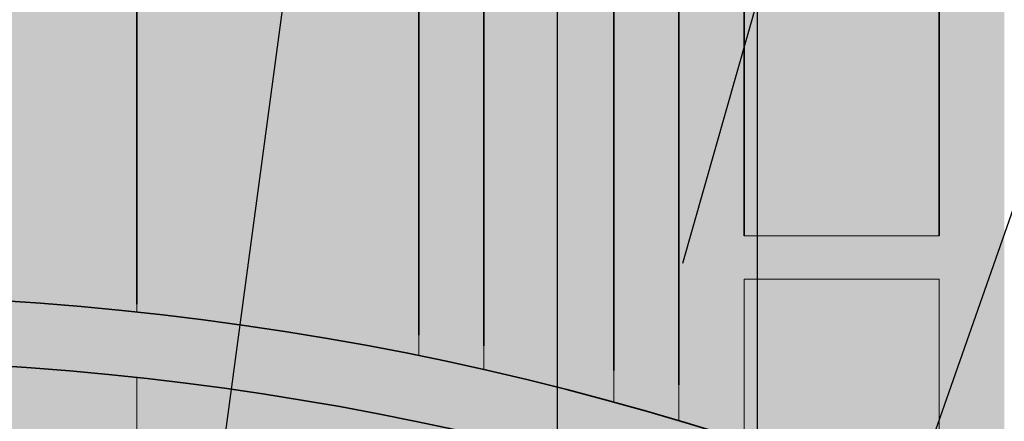
# Model space of a CAD drawing. Units: millimetres. Extents: x 130 to 1021, y 147 to 699.
# Tile 27 of 40: x 442 to 487, y 505 to 524. Entities that reach past the tile are written whole.
import ezdxf

# ---------------------------------------------------------------- set-up
doc = ezdxf.new("R2010")
doc.units = ezdxf.units.MM
doc.header["$MEASUREMENT"] = 0
for name, color, linetype, lineweight in [('A-ANNO-DIMS', 2, 'Continuous', 18), ('A-ELEV', 7, 'Continuous', 35), ('A-ELEV-PATT', 9, 'Continuous', 13), ('A-ELEV-RAIL', 6, 'Continuous', 18)]:
    doc.layers.add(name, color=color, linetype=linetype, lineweight=lineweight)
doc.styles.get("Standard").update_dxf_attribs({"font": 'arial.ttf'})
doc.dimstyles.get("Standard").update_dxf_attribs({"dimtxt": 20, "dimasz": 10, "dimexe": 10, "dimexo": 10, "dimgap": 5, "dimtad": 0, "dimtih": 1, "dimtoh": 1, "dimdec": 0, "dimzin": 0, "dimdsep": 46, "dimtxsty": 'Standard', "dimcen": 5, "dimadec": 0, "dimazin": 0, "dimtfac": 1, "dimtdec": 0, "dimtofl": 0, "dimtmove": 0, "dimatfit": 3, "dimfxl": 1, "dimtolj": 1, "dimtzin": 0, "dimarcsym": 0})

# ---------------------------------------------------------------- blocks, each defined once
blk = doc.blocks.new('*D11')
at = {"layer": 'A-ANNO-DIMS', "color": 0, "lineweight": -2, "transparency": 16777216}
for p, q in [((737.374, 648.699), (737.374, 149.739)), ((299.374, 566.947), (299.374, 149.739)), ((309.374, 159.739), (490.857, 159.739)), ((727.374, 159.739), (545.891, 159.739))]:
    blk.add_line(p, q, dxfattribs=at)
at = {"layer": 'A-ANNO-DIMS', "color": 0, "transparency": 16777216}
for points in [[(309.374, 161.406), (309.374, 158.073), (299.374, 159.739)], [(727.374, 161.406), (727.374, 158.073), (737.374, 159.739)]]:
    blk.add_solid(points, dxfattribs=at)
at = {"layer": 'Defpoints', "color": 0, "transparency": 16777216}
for p in [(737.374, 658.699), (299.374, 576.947), (737.374, 159.739)]:
    blk.add_point(p, dxfattribs=at)
at = {"layer": 'A-ANNO-DIMS', "color": 0, "transparency": 16777216, "insert": (518.374, 159.739), "char_height": 20, "attachment_point": 5}
blk.add_mtext('\\A1;438', dxfattribs=at)
blk = doc.blocks.new('*D12')
at = {"layer": 'A-ANNO-DIMS', "color": 0, "lineweight": -2, "transparency": 16777216}
for p, q in [((477.374, 661.947), (265.074, 661.947)), ((275.074, 651.947), (275.074, 438.205)), ((275.074, 194.039), (275.074, 407.782)), ((357.163, 184.039), (265.074, 184.039))]:
    blk.add_line(p, q, dxfattribs=at)
at = {"layer": 'A-ANNO-DIMS', "color": 0, "transparency": 16777216}
for points in [[(273.407, 651.947), (276.74, 651.947), (275.074, 661.947)], [(273.407, 194.039), (276.74, 194.039), (275.074, 184.039)]]:
    blk.add_solid(points, dxfattribs=at)
at = {"layer": 'Defpoints', "color": 0, "transparency": 16777216}
for p in [(275.074, 661.947), (487.374, 661.947), (367.163, 184.039)]:
    blk.add_point(p, dxfattribs=at)
at = {"layer": 'A-ANNO-DIMS', "color": 0, "transparency": 16777216, "insert": (275.074, 422.993), "char_height": 20, "attachment_point": 5}
blk.add_mtext('\\A1;477.9', dxfattribs=at)
blk = doc.blocks.new('*D16')
at = {"layer": 'A-ANNO-DIMS', "color": 0, "lineweight": -2, "transparency": 16777216}
for p, q in [((357.941, 411.947), (357.941, 696.247)), ((363.922, 579.884), (363.922, 696.247)), ((347.941, 686.247), (337.941, 686.247)), ((373.922, 686.247), (383.922, 686.247))]:
    blk.add_line(p, q, dxfattribs=at)
at = {"layer": 'A-ANNO-DIMS', "color": 0, "transparency": 16777216}
for points in [[(347.941, 687.914), (347.941, 684.581), (357.941, 686.247)], [(373.922, 687.914), (373.922, 684.581), (363.922, 686.247)]]:
    blk.add_solid(points, dxfattribs=at)
at = {"layer": 'Defpoints', "color": 0, "transparency": 16777216}
for p in [(363.922, 686.247), (363.922, 569.884), (357.941, 401.947)]:
    blk.add_point(p, dxfattribs=at)
at = {"layer": 'A-ANNO-DIMS', "color": 0, "transparency": 16777216, "insert": (420.737, 686.247), "char_height": 20, "attachment_point": 5}
blk.add_mtext('\\A1;5.981', dxfattribs=at)
blk = doc.blocks.new('*D17')
at = {"layer": 'A-ANNO-DIMS', "color": 0, "lineweight": -2, "transparency": 16777216}
for p, q in [((363.922, 579.884), (363.922, 696.247)), ((375.85, 490.216), (375.85, 696.247)), ((353.922, 686.247), (343.922, 686.247)), ((385.85, 686.247), (395.85, 686.247))]:
    blk.add_line(p, q, dxfattribs=at)
at = {"layer": 'A-ANNO-DIMS', "color": 0, "transparency": 16777216}
for points in [[(353.922, 687.914), (353.922, 684.581), (363.922, 686.247)], [(385.85, 687.914), (385.85, 684.581), (375.85, 686.247)]]:
    blk.add_solid(points, dxfattribs=at)
at = {"layer": 'Defpoints', "color": 0, "transparency": 16777216}
for p in [(375.85, 686.247), (363.922, 569.884), (375.85, 480.216)]:
    blk.add_point(p, dxfattribs=at)
at = {"layer": 'A-ANNO-DIMS', "color": 0, "transparency": 16777216, "insert": (441.444, 686.247), "char_height": 20, "attachment_point": 5}
blk.add_mtext('\\A1;11.928', dxfattribs=at)
blk = doc.blocks.new('*D18')
at = {"layer": 'A-ANNO-DIMS', "color": 0, "lineweight": -2, "transparency": 16777216}
for p, q in [((375.85, 490.216), (375.85, 696.247)), ((382.374, 388.947), (382.374, 696.247)), ((365.85, 686.247), (355.85, 686.247)), ((392.374, 686.247), (402.374, 686.247))]:
    blk.add_line(p, q, dxfattribs=at)
at = {"layer": 'A-ANNO-DIMS', "color": 0, "transparency": 16777216}
for points in [[(365.85, 687.914), (365.85, 684.581), (375.85, 686.247)], [(392.374, 687.914), (392.374, 684.581), (382.374, 686.247)]]:
    blk.add_solid(points, dxfattribs=at)
at = {"layer": 'Defpoints', "color": 0, "transparency": 16777216}
for p in [(382.374, 686.247), (375.85, 480.216), (382.374, 378.947)]:
    blk.add_point(p, dxfattribs=at)
at = {"layer": 'A-ANNO-DIMS', "color": 0, "transparency": 16777216, "insert": (441.132, 686.247), "char_height": 20, "attachment_point": 5}
blk.add_mtext('\\A1;6.524', dxfattribs=at)
blk = doc.blocks.new('*D19')
at = {"layer": 'A-ANNO-DIMS', "color": 0, "lineweight": -2, "transparency": 16777216}
for p, q in [((382.374, 388.947), (382.374, 696.247)), ((414.652, 510.881), (414.652, 696.247)), ((392.374, 686.247), (404.652, 686.247)), ((414.652, 686.247), (424.652, 686.247))]:
    blk.add_line(p, q, dxfattribs=at)
at = {"layer": 'A-ANNO-DIMS', "color": 0, "transparency": 16777216}
for points in [[(392.374, 687.914), (392.374, 684.581), (382.374, 686.247)], [(404.652, 687.914), (404.652, 684.581), (414.652, 686.247)]]:
    blk.add_solid(points, dxfattribs=at)
at = {"layer": 'Defpoints', "color": 0, "transparency": 16777216}
for p in [(414.652, 686.247), (414.652, 500.881), (382.374, 378.947)]:
    blk.add_point(p, dxfattribs=at)
at = {"layer": 'A-ANNO-DIMS', "color": 0, "transparency": 16777216, "insert": (463.411, 686.247), "char_height": 20, "attachment_point": 5}
blk.add_mtext('\\A1;32.28', dxfattribs=at)
blk = doc.blocks.new('*D20')
at = {"layer": 'A-ANNO-DIMS', "color": 0, "lineweight": -2, "transparency": 16777216}
for p, q in [((414.652, 510.881), (414.652, 696.247)), ((432.374, 388.947), (432.374, 696.247)), ((404.652, 686.247), (394.652, 686.247)), ((442.374, 686.247), (452.374, 686.247))]:
    blk.add_line(p, q, dxfattribs=at)
at = {"layer": 'A-ANNO-DIMS', "color": 0, "transparency": 16777216}
for points in [[(404.652, 687.914), (404.652, 684.581), (414.652, 686.247)], [(442.374, 687.914), (442.374, 684.581), (432.374, 686.247)]]:
    blk.add_solid(points, dxfattribs=at)
at = {"layer": 'Defpoints', "color": 0, "transparency": 16777216}
for p in [(432.374, 686.247), (414.652, 500.881), (432.374, 378.947)]:
    blk.add_point(p, dxfattribs=at)
at = {"layer": 'A-ANNO-DIMS', "color": 0, "transparency": 16777216, "insert": (490.075, 686.247), "char_height": 20, "attachment_point": 5}
blk.add_mtext('\\A1;17.72', dxfattribs=at)
blk = doc.blocks.new('*D21')
at = {"layer": 'A-ANNO-DIMS', "color": 0, "lineweight": -2, "transparency": 16777216}
for p, q in [((432.374, 388.947), (432.374, 696.247)), ((447.374, 656.947), (447.374, 696.247)), ((422.374, 686.247), (412.374, 686.247)), ((457.374, 686.247), (467.374, 686.247))]:
    blk.add_line(p, q, dxfattribs=at)
at = {"layer": 'A-ANNO-DIMS', "color": 0, "transparency": 16777216}
for points in [[(422.374, 687.914), (422.374, 684.581), (432.374, 686.247)], [(457.374, 687.914), (457.374, 684.581), (447.374, 686.247)]]:
    blk.add_solid(points, dxfattribs=at)
at = {"layer": 'Defpoints', "color": 0, "transparency": 16777216}
for p in [(447.374, 686.247), (447.374, 646.947), (432.374, 378.947)]:
    blk.add_point(p, dxfattribs=at)
at = {"layer": 'A-ANNO-DIMS', "color": 0, "transparency": 16777216, "insert": (485.832, 686.247), "char_height": 20, "attachment_point": 5}
blk.add_mtext('\\A1;15', dxfattribs=at)
blk = doc.blocks.new('*D22')
at = {"layer": 'A-ANNO-DIMS', "color": 0, "lineweight": -2, "transparency": 16777216}
for p, q in [((447.374, 656.947), (447.374, 696.247)), ((466.767, 403.947), (466.767, 696.247)), ((437.374, 686.247), (427.374, 686.247)), ((476.767, 686.247), (486.767, 686.247))]:
    blk.add_line(p, q, dxfattribs=at)
at = {"layer": 'A-ANNO-DIMS', "color": 0, "transparency": 16777216}
for points in [[(437.374, 687.914), (437.374, 684.581), (447.374, 686.247)], [(476.767, 687.914), (476.767, 684.581), (466.767, 686.247)]]:
    blk.add_solid(points, dxfattribs=at)
at = {"layer": 'Defpoints', "color": 0, "transparency": 16777216}
for p in [(466.767, 686.247), (447.374, 646.947), (466.767, 393.947)]:
    blk.add_point(p, dxfattribs=at)
at = {"layer": 'A-ANNO-DIMS', "color": 0, "transparency": 16777216, "insert": (532.34, 686.247), "char_height": 20, "attachment_point": 5}
blk.add_mtext('\\A1;19.393', dxfattribs=at)
blk = doc.blocks.new('*D23')
at = {"layer": 'A-ANNO-DIMS', "color": 0, "lineweight": -2, "transparency": 16777216}
for p, q in [((466.767, 403.947), (466.767, 696.247)), ((475.988, 209.039), (475.988, 696.247)), ((456.767, 686.247), (446.767, 686.247)), ((485.988, 686.247), (495.988, 686.247))]:
    blk.add_line(p, q, dxfattribs=at)
at = {"layer": 'A-ANNO-DIMS', "color": 0, "transparency": 16777216}
for points in [[(456.767, 687.914), (456.767, 684.581), (466.767, 686.247)], [(485.988, 687.914), (485.988, 684.581), (475.988, 686.247)]]:
    blk.add_solid(points, dxfattribs=at)
at = {"layer": 'Defpoints', "color": 0, "transparency": 16777216}
for p in [(475.988, 686.247), (466.767, 393.947), (475.988, 199.039)]:
    blk.add_point(p, dxfattribs=at)
at = {"layer": 'A-ANNO-DIMS', "color": 0, "transparency": 16777216, "insert": (534.631, 686.247), "char_height": 20, "attachment_point": 5}
blk.add_mtext('\\A1;9.222', dxfattribs=at)
blk = doc.blocks.new('*D24')
at = {"layer": 'A-ANNO-DIMS', "color": 0, "lineweight": -2, "transparency": 16777216}
for p, q in [((475.988, 209.039), (475.988, 696.247)), ((487.374, 671.947), (487.374, 696.247)), ((465.988, 686.247), (455.988, 686.247)), ((497.374, 686.247), (507.374, 686.247))]:
    blk.add_line(p, q, dxfattribs=at)
at = {"layer": 'A-ANNO-DIMS', "color": 0, "transparency": 16777216}
for points in [[(465.988, 687.914), (465.988, 684.581), (475.988, 686.247)], [(497.374, 687.914), (497.374, 684.581), (487.374, 686.247)]]:
    blk.add_solid(points, dxfattribs=at)
at = {"layer": 'Defpoints', "color": 0, "transparency": 16777216}
for p in [(487.374, 686.247), (487.374, 661.947), (475.988, 199.039)]:
    blk.add_point(p, dxfattribs=at)
at = {"layer": 'A-ANNO-DIMS', "color": 0, "transparency": 16777216, "insert": (553.022, 686.247), "char_height": 20, "attachment_point": 5}
blk.add_mtext('\\A1;11.385', dxfattribs=at)
blk = doc.blocks.new('*D25')
at = {"layer": 'A-ANNO-DIMS', "color": 0, "lineweight": -2, "transparency": 16777216}
for p, q in [((487.374, 671.947), (487.374, 696.247)), ((494.102, 506.908), (494.102, 696.247)), ((477.374, 686.247), (467.374, 686.247)), ((504.102, 686.247), (514.102, 686.247))]:
    blk.add_line(p, q, dxfattribs=at)
at = {"layer": 'A-ANNO-DIMS', "color": 0, "transparency": 16777216}
for points in [[(477.374, 687.914), (477.374, 684.581), (487.374, 686.247)], [(504.102, 687.914), (504.102, 684.581), (494.102, 686.247)]]:
    blk.add_solid(points, dxfattribs=at)
at = {"layer": 'Defpoints', "color": 0, "transparency": 16777216}
for p in [(494.102, 686.247), (487.374, 661.947), (494.102, 496.908)]:
    blk.add_point(p, dxfattribs=at)
at = {"layer": 'A-ANNO-DIMS', "color": 0, "transparency": 16777216, "insert": (552.922, 686.247), "char_height": 20, "attachment_point": 5}
blk.add_mtext('\\A1;6.728', dxfattribs=at)
blk = doc.blocks.new('*D26')
at = {"layer": 'A-ANNO-DIMS', "color": 0, "lineweight": -2, "transparency": 16777216}
for p, q in [((494.102, 506.908), (494.102, 696.247)), ((502.374, 593.947), (502.374, 696.247)), ((484.102, 686.247), (474.102, 686.247)), ((512.374, 686.247), (522.374, 686.247))]:
    blk.add_line(p, q, dxfattribs=at)
at = {"layer": 'A-ANNO-DIMS', "color": 0, "transparency": 16777216}
for points in [[(484.102, 687.914), (484.102, 684.581), (494.102, 686.247)], [(512.374, 687.914), (512.374, 684.581), (502.374, 686.247)]]:
    blk.add_solid(points, dxfattribs=at)
at = {"layer": 'Defpoints', "color": 0, "transparency": 16777216}
for p in [(502.374, 686.247), (502.374, 583.947), (494.102, 496.908)]:
    blk.add_point(p, dxfattribs=at)
at = {"layer": 'A-ANNO-DIMS', "color": 0, "transparency": 16777216, "insert": (561.03, 686.247), "char_height": 20, "attachment_point": 5}
blk.add_mtext('\\A1;8.272', dxfattribs=at)
blk = doc.blocks.new('*D65')
at = {"layer": 'A-ANNO-DIMS', "color": 0, "lineweight": -2, "transparency": 16777216}
for p, q in [((495.463, 509.127), (472.508, 423.108)), ((505.463, 509.127), (495.463, 509.127)), ((427.374, 248.979), (427.374, 258.979)), ((422.374, 253.979), (432.374, 253.979))]:
    blk.add_line(p, q, dxfattribs=at)
at = {"layer": 'A-ANNO-DIMS', "color": 0, "transparency": 16777216}
blk.add_solid([(470.898, 423.538), (474.118, 422.679), (469.93, 413.447)], dxfattribs=at)
at = {"layer": 'Defpoints', "color": 0, "transparency": 16777216}
for p in [(469.93, 413.447), (427.374, 253.979)]:
    blk.add_point(p, dxfattribs=at)
at = {"layer": 'A-ANNO-DIMS', "color": 0, "transparency": 16777216, "insert": (561.623, 509.127), "char_height": 20, "attachment_point": 5}
blk.add_mtext('\\A1;R165.05', dxfattribs=at)
blk = doc.blocks.new('*D67')
at = {"layer": 'A-ANNO-DIMS', "color": 0, "lineweight": -2, "transparency": 16777216}
for p, q in [((479.756, 492.431), (462.144, 412.223)), ((489.756, 492.431), (479.756, 492.431)), ((427.07, 247.496), (427.07, 257.496)), ((422.07, 252.496), (432.07, 252.496))]:
    blk.add_line(p, q, dxfattribs=at)
at = {"layer": 'A-ANNO-DIMS', "color": 0, "transparency": 16777216}
blk.add_solid([(460.516, 412.58), (463.772, 411.865), (459.999, 402.455)], dxfattribs=at)
at = {"layer": 'Defpoints', "color": 0, "transparency": 16777216}
for p in [(459.999, 402.455), (427.07, 252.496)]:
    blk.add_point(p, dxfattribs=at)
at = {"layer": 'A-ANNO-DIMS', "color": 0, "transparency": 16777216, "insert": (545.841, 492.431), "char_height": 20, "attachment_point": 5}
blk.add_mtext('\\A1;R153.53', dxfattribs=at)
blk = doc.blocks.new('*D69')
at = {"layer": 'A-ANNO-DIMS', "color": 0, "lineweight": -2, "transparency": 16777216}
for p, q in [((507.746, 572.261), (483.091, 501.813)), ((517.746, 572.261), (507.746, 572.261)), ((433.191, 354.23), (433.191, 364.23)), ((428.191, 359.23), (438.191, 359.23))]:
    blk.add_line(p, q, dxfattribs=at)
at = {"layer": 'A-ANNO-DIMS', "color": 0, "transparency": 16777216}
blk.add_solid([(481.518, 502.363), (484.664, 501.262), (479.788, 492.374)], dxfattribs=at)
at = {"layer": 'Defpoints', "color": 0, "transparency": 16777216}
for p in [(479.788, 492.374), (433.191, 359.23)]:
    blk.add_point(p, dxfattribs=at)
at = {"layer": 'A-ANNO-DIMS', "color": 0, "transparency": 16777216, "insert": (573.824, 572.261), "char_height": 20, "attachment_point": 5}
blk.add_mtext('\\A1;R141.06', dxfattribs=at)
blk = doc.blocks.new('*D71')
at = {"layer": 'A-ANNO-DIMS', "color": 0, "lineweight": -2, "transparency": 16777216}
for p, q in [((492.108, 581.609), (472.542, 512.666)), ((502.108, 581.609), (492.108, 581.609)), ((432.65, 367.109), (432.65, 377.109)), ((427.65, 372.109), (437.65, 372.109))]:
    blk.add_line(p, q, dxfattribs=at)
at = {"layer": 'A-ANNO-DIMS', "color": 0, "transparency": 16777216}
blk.add_solid([(470.938, 513.121), (474.145, 512.211), (469.812, 503.046)], dxfattribs=at)
at = {"layer": 'Defpoints', "color": 0, "transparency": 16777216}
for p in [(469.812, 503.046), (432.65, 372.109)]:
    blk.add_point(p, dxfattribs=at)
at = {"layer": 'A-ANNO-DIMS', "color": 0, "transparency": 16777216, "insert": (548.493, 581.609), "char_height": 20, "attachment_point": 5}
blk.add_mtext('\\A1;R136.1', dxfattribs=at)
blk = doc.blocks.new('*D72')
at = {"layer": 'A-ANNO-DIMS', "color": 0, "lineweight": -2, "transparency": 16777216}
for p, q in [((460.658, 573.64), (451.279, 503.49)), ((470.658, 573.64), (460.658, 573.64)), ((432.115, 355.142), (432.115, 365.142)), ((427.115, 360.142), (437.115, 360.142))]:
    blk.add_line(p, q, dxfattribs=at)
at = {"layer": 'A-ANNO-DIMS', "color": 0, "transparency": 16777216}
blk.add_solid([(449.628, 503.711), (452.931, 503.27), (449.954, 493.579)], dxfattribs=at)
at = {"layer": 'Defpoints', "color": 0, "transparency": 16777216}
for p in [(449.954, 493.579), (432.115, 360.142)]:
    blk.add_point(p, dxfattribs=at)
at = {"layer": 'A-ANNO-DIMS', "color": 0, "transparency": 16777216, "insert": (526.64, 573.64), "char_height": 20, "attachment_point": 5}
blk.add_mtext('\\A1;R134.62', dxfattribs=at)

msp = doc.modelspace()

# ---------------------------------------------------------------- hatches: boundary and pattern name
at = {"layer": 'A-ELEV-PATT'}
h = msp.add_hatch(color=256, dxfattribs=at)
h.dxf.hatch_style = 1
h.paths.add_polyline_path([(737.3738, 658.6988, 0.0135961), (632.4019, 661.9473), (607.3738, 661.9473), (487.3738, 661.9473), (487.3738, 649.9473), (607.3738, 649.9473), (632.3794, 649.9473, -0.0136841), (737.3738, 646.6784)])
h.paths.add_polyline_path([(732.3738, 643.9599, 0.0130529), (632.3738, 646.9473), (607.3738, 646.9473), (487.3738, 646.9473), (487.3738, 596.9473), (632.3738, 596.9473, -0.0130529), (732.3738, 593.9599)])
h.paths.add_polyline_path([(737.3738, 593.6732, 0.0137063), (632.3738, 596.9473), (487.3738, 596.9473), (487.3738, 586.9473), (632.355, 586.9473, -0.0137808), (737.3738, 583.6559)])
h.paths.add_polyline_path([(447.3738, 646.9473), (307.3738, 646.9473), (302.3738, 646.9473), (302.3738, 634.9473), (447.3738, 634.9473)])
h.paths.add_polyline_path([(447.3738, 631.9473), (307.3738, 631.9473), (307.3738, 586.9473), (447.3738, 586.9473)])
h.paths.add_polyline_path([(447.3738, 586.9473), (307.3738, 586.9473), (302.3738, 586.9473), (302.3738, 576.9473), (447.3738, 576.9473)])
h.paths.add_polyline_path([(447.3738, 573.9473), (367.3738, 573.9473), (367.3738, 539.9473), (447.3738, 539.9473)])
h.paths.add_polyline_path([(447.3738, 537.9473), (367.3738, 537.9473), (367.3738, 507.9473), (400.392, 507.4253, -0.001728), (401.3281, 507.6451, -0.5220025), (425.6117, 511.0391, -0.0391849), (447.3738, 510.4359), (447.3738, 510.7883)])
h.paths.add_polyline_path([(394.7238, 505.9473), (367.3738, 505.9473), (367.3738, 476.9473, -0.0146512), (375.8501, 480.2159), (376.1506, 499.2266, -0.0355419)])
h.paths.add_polyline_path([(632.3738, 583.9473), (552.3738, 583.9473), (552.3738, 550.9473), (632.3738, 550.9473)])
h.paths.add_polyline_path([(632.3738, 548.9473), (552.3738, 548.9473), (552.3738, 515.9473), (632.3738, 515.9473)])
h.paths.add_polyline_path([(632.3738, 513.9473), (552.3738, 513.9473), (552.3738, 476.9473), (632.3738, 476.9473)])
h.paths.add_polyline_path([(737.3738, 473.6903, 0.0136326), (632.3926, 476.9473), (552.3738, 476.9473), (487.3738, 476.9473), (487.3738, 466.9473), (632.3738, 466.9473, -0.0137063), (737.3738, 463.6732)])
h.paths.add_polyline_path([(732.3738, 460.9552, 0.0130741), (632.3681, 463.9473), (487.3738, 463.9473), (487.3738, 407.735, -0.0032286), (489.3544, 406.9473), (632.3926, 406.9473, -0.0129826), (732.3738, 403.9755)])
h.paths.add_polyline_path([(487.3738, 463.9473, 0.20133), (367.3738, 463.9473), (367.3738, 407.735, -0.1882031), (487.3738, 407.735)])
h.paths.add_polyline_path([(367.3738, 476.9473), (367.3738, 466.9473, -0.2013309), (487.3738, 466.9473), (487.3738, 476.9473, 0.20133)])
h.paths.add_polyline_path([(367.3738, 463.9473), (307.3738, 463.9473), (307.3738, 401.9473), (357.9413, 401.9473), (367.3738, 407.735)])
h.paths.add_polyline_path([(367.3738, 476.9473), (302.3738, 476.9473), (302.3738, 466.9473), (367.3738, 466.9473)])
h.paths.add_polyline_path([(632.8184, 366.9453), (552.3738, 366.9453), (552.3738, 393.9473), (632.8184, 393.9473)])
h.paths.add_polyline_path([(632.8184, 357.2114), (632.8184, 363.9453), (552.3738, 363.9453), (552.3738, 357.2114), (552.3738, 336.9453), (632.8184, 336.9453)])
h.paths.add_polyline_path([(632.8184, 333.9453), (552.3738, 333.9453), (552.3738, 306.9453), (632.8184, 306.9453)])
h.paths.add_polyline_path([(632.8184, 303.9453), (552.3738, 303.9453), (552.3738, 273.9473), (632.355, 273.9473, 0.0000608), (632.8184, 273.9491)])
h.paths.add_polyline_path([(737.3738, 403.6903, 0.0136326), (632.3926, 406.9473), (489.3544, 406.9473, 0.1915481), (367.3738, 407.735), (367.3738, 396.9473, -0.2013309), (487.3738, 396.9473), (632.3738, 396.9473, -0.0137063), (737.3738, 393.6732)])
h.paths.add_polyline_path([(357.9413, 401.9473), (307.3738, 401.9473), (307.3738, 391.9473), (357.9413, 391.9473)])
h.paths.add_polyline_path([(357.9413, 357.2114), (357.9413, 388.9473), (307.3738, 388.9473), (307.3738, 357.2114), (307.3738, 273.9473), (357.9413, 273.9473)])
h.paths.add_polyline_path([(732.3738, 263.93, -0.0130317), (632.3794, 260.9473), (466.7667, 260.9473), (466.7667, 240.9473), (469.8406, 236.978), (469.8406, 221.978), (472.9145, 218.0087), (472.9145, 213.9473), (607.3738, 213.9473), (732.3738, 213.9473)])
h.paths.add_polyline_path([(732.3738, 290.889), (722.479, 290.889), (722.479, 301.889), (732.3738, 301.889), (732.3738, 305.889), (722.479, 305.889), (722.479, 316.889), (732.3738, 316.889), (732.3738, 320.889), (722.479, 320.889), (722.479, 331.889), (732.3738, 331.889), (732.3738, 335.889), (722.479, 335.889), (722.479, 346.889), (732.3738, 346.889), (732.3738, 350.889), (722.479, 350.889), (722.479, 361.889), (732.3738, 361.889), (732.3738, 365.889), (722.479, 365.889), (722.479, 376.889), (732.3738, 376.889), (732.3738, 380.889), (722.479, 380.889), (722.479, 391.4848, 0.0005233), (718.479, 391.6843), (718.479, 380.889), (707.479, 380.889), (707.479, 392.1896, 0.0005231), (703.479, 392.3576), (703.479, 380.889), (692.479, 380.889), (692.479, 392.7765, 0.0005229), (688.479, 392.9131), (688.479, 380.889), (677.479, 380.889), (677.479, 393.2456, 0.0005228), (673.479, 393.3508), (673.479, 380.889), (662.479, 380.889), (662.479, 393.597, 0.0005227), (658.479, 393.6709), (658.479, 380.889), (647.479, 380.889), (647.479, 393.8308, 0.0005226), (643.479, 393.8732), (643.479, 380.889), (632.8184, 380.889), (632.8184, 376.889), (643.479, 376.889), (643.479, 365.889), (632.8184, 365.889), (632.8184, 361.889), (643.479, 361.889), (643.479, 350.889), (632.8184, 350.889), (632.8184, 346.889), (643.479, 346.889), (643.479, 335.889), (632.8184, 335.889), (632.8184, 331.889), (643.479, 331.889), (643.479, 320.889), (632.8184, 320.889), (632.8184, 316.889), (643.479, 316.889), (643.479, 305.889), (632.8184, 305.889), (632.8184, 301.889), (643.479, 301.889), (643.479, 290.889), (632.8184, 290.889), (632.8184, 286.889), (643.479, 286.889), (643.479, 274.0217, 0.0005246), (647.479, 274.0643), (647.479, 286.889), (658.479, 286.889), (658.479, 274.2248, 0.0005246), (662.479, 274.2989), (662.479, 286.889), (673.479, 286.889), (673.479, 274.546, 0.0005247), (677.479, 274.6516), (677.479, 286.889), (688.479, 286.889), (688.479, 274.9853, 0.0005248), (692.479, 275.1224), (692.479, 286.889), (703.479, 286.889), (703.479, 275.5429, 0.000525), (707.479, 275.7115), (707.479, 286.889), (718.479, 286.889), (718.479, 276.2187, 0.0005252), (722.479, 276.4189), (722.479, 286.889), (732.3738, 286.889)])
h.paths.add_polyline_path([(718.479, 290.889), (707.479, 290.889), (707.479, 301.889), (718.479, 301.889)], flags=16)
h.paths.add_polyline_path([(703.479, 290.889), (692.479, 290.889), (692.479, 301.889), (703.479, 301.889)], flags=16)
h.paths.add_polyline_path([(718.479, 305.889), (707.479, 305.889), (707.479, 316.889), (718.479, 316.889)], flags=16)
h.paths.add_polyline_path([(703.479, 305.889), (692.479, 305.889), (692.479, 316.889), (703.479, 316.889)], flags=16)
h.paths.add_polyline_path([(688.479, 290.889), (677.479, 290.889), (677.479, 301.889), (688.479, 301.889)], flags=16)
h.paths.add_polyline_path([(718.479, 320.889), (707.479, 320.889), (707.479, 331.889), (718.479, 331.889)], flags=16)
h.paths.add_polyline_path([(688.479, 305.889), (677.479, 305.889), (677.479, 316.889), (688.479, 316.889)], flags=16)
h.paths.add_polyline_path([(703.479, 320.889), (692.479, 320.889), (692.479, 331.889), (703.479, 331.889)], flags=16)
h.paths.add_polyline_path([(688.479, 320.889), (677.479, 320.889), (677.479, 331.889), (688.479, 331.889)], flags=16)
h.paths.add_polyline_path([(673.479, 290.889), (662.479, 290.889), (662.479, 301.889), (673.479, 301.889)], flags=16)
h.paths.add_polyline_path([(718.479, 335.889), (707.479, 335.889), (707.479, 346.889), (718.479, 346.889)], flags=16)
h.paths.add_polyline_path([(673.479, 305.889), (662.479, 305.889), (662.479, 316.889), (673.479, 316.889)], flags=16)
h.paths.add_polyline_path([(703.479, 335.889), (692.479, 335.889), (692.479, 346.889), (703.479, 346.889)], flags=16)
h.paths.add_polyline_path([(673.479, 320.889), (662.479, 320.889), (662.479, 331.889), (673.479, 331.889)], flags=16)
h.paths.add_polyline_path([(688.479, 335.889), (677.479, 335.889), (677.479, 346.889), (688.479, 346.889)], flags=16)
h.paths.add_polyline_path([(658.479, 290.889), (647.479, 290.889), (647.479, 301.889), (658.479, 301.889)], flags=16)
h.paths.add_polyline_path([(718.479, 350.889), (707.479, 350.889), (707.479, 361.889), (718.479, 361.889)], flags=16)
h.paths.add_polyline_path([(658.479, 305.889), (647.479, 305.889), (647.479, 316.889), (658.479, 316.889)], flags=16)
h.paths.add_polyline_path([(703.479, 350.889), (692.479, 350.889), (692.479, 361.889), (703.479, 361.889)], flags=16)
h.paths.add_polyline_path([(673.479, 335.889), (662.479, 335.889), (662.479, 346.889), (673.479, 346.889)], flags=16)
h.paths.add_polyline_path([(658.479, 320.889), (647.479, 320.889), (647.479, 331.889), (658.479, 331.889)], flags=16)
h.paths.add_polyline_path([(688.479, 350.889), (677.479, 350.889), (677.479, 361.889), (688.479, 361.889)], flags=16)
h.paths.add_polyline_path([(718.479, 365.889), (707.479, 365.889), (707.479, 376.889), (718.479, 376.889)], flags=16)
h.paths.add_polyline_path([(658.479, 335.889), (647.479, 335.889), (647.479, 346.889), (658.479, 346.889)], flags=16)
h.paths.add_polyline_path([(673.479, 350.889), (662.479, 350.889), (662.479, 361.889), (673.479, 361.889)], flags=16)
h.paths.add_polyline_path([(703.479, 365.889), (692.479, 365.889), (692.479, 376.889), (703.479, 376.889)], flags=16)
h.paths.add_polyline_path([(688.479, 365.889), (677.479, 365.889), (677.479, 376.889), (688.479, 376.889)], flags=16)
h.paths.add_polyline_path([(658.479, 350.889), (647.479, 350.889), (647.479, 361.889), (658.479, 361.889)], flags=16)
h.paths.add_polyline_path([(673.479, 365.889), (662.479, 365.889), (662.479, 376.889), (673.479, 376.889)], flags=16)
h.paths.add_polyline_path([(658.479, 365.889), (647.479, 365.889), (647.479, 376.889), (658.479, 376.889)], flags=16)
h.paths.add_polyline_path([(732.3738, 503.9786), (722.3392, 503.9786), (722.3392, 514.9786), (732.3738, 514.9786), (732.3738, 518.9786), (722.3392, 518.9786), (722.3392, 529.9786), (732.3738, 529.9786), (732.3738, 533.9786), (722.3392, 533.9786), (722.3392, 544.9786), (732.3738, 544.9786), (732.3738, 546.9473), (732.3738, 548.9786), (722.3392, 548.9786), (722.3392, 559.9786), (732.3738, 559.9786), (732.3738, 563.9786), (722.3392, 563.9786), (722.3392, 574.9786), (732.3738, 574.9786), (732.3738, 578.9786), (722.3392, 578.9786), (722.3392, 581.4789, 0.000526), (718.3392, 581.6791), (718.3392, 578.9786), (707.3392, 578.9786), (707.3392, 582.1863, 0.0005258), (703.3392, 582.355), (703.3392, 578.9786), (692.3392, 578.9786), (692.3392, 582.7752, 0.0005257), (688.3392, 582.9123), (688.3392, 578.9786), (677.3392, 578.9786), (677.3392, 583.2457, 0.0005255), (673.3392, 583.3512), (673.3392, 578.9786), (662.3392, 578.9786), (662.3392, 583.5978, 0.0005254), (658.3392, 583.6718), (658.3392, 578.9786), (647.3392, 578.9786), (647.3392, 583.8317, 0.0005254), (643.3392, 583.8741), (643.3392, 578.9786), (632.3738, 578.9786), (632.3738, 574.9786), (643.3392, 574.9786), (643.3392, 563.9786), (632.3738, 563.9786), (632.3738, 559.9786), (643.3392, 559.9786), (643.3392, 548.9786), (632.3738, 548.9786), (632.3738, 544.9786), (643.3392, 544.9786), (643.3392, 533.9786), (632.3738, 533.9786), (632.3738, 529.9786), (643.3392, 529.9786), (643.3392, 518.9786), (632.3738, 518.9786), (632.3738, 515.9473), (632.3738, 514.9786), (643.3392, 514.9786), (643.3392, 503.9786), (632.3738, 503.9786), (632.3738, 499.9786), (643.3392, 499.9786), (643.3392, 488.9786), (632.3738, 488.9786), (632.3738, 484.9786), (643.3392, 484.9786), (643.3392, 476.8751, -0.0005191), (647.3392, 476.8332), (647.3392, 484.9786), (658.3392, 484.9786), (658.3392, 476.6752, -0.0005192), (662.3392, 476.6022), (662.3392, 484.9786), (673.3392, 484.9786), (673.3392, 476.3585, -0.0005193), (677.3392, 476.2543), (677.3392, 484.9786), (688.3392, 484.9786), (688.3392, 475.9248, -0.0005194), (692.3392, 475.7894), (692.3392, 484.9786), (703.3392, 484.9786), (703.3392, 475.3741, -0.0005195), (707.3392, 475.2075), (707.3392, 484.9786), (718.3392, 484.9786), (718.3392, 474.7064, -0.0005197), (722.3392, 474.5086), (722.3392, 484.9786), (732.3738, 484.9786), (732.3738, 488.9786), (722.3392, 488.9786), (722.3392, 499.9786), (732.3738, 499.9786)])
h.paths.add_polyline_path([(718.3392, 503.9786), (707.3392, 503.9786), (707.3392, 514.9786), (718.3392, 514.9786)], flags=16)
h.paths.add_polyline_path([(718.3392, 499.9786), (718.3392, 488.9786), (707.3392, 488.9786), (707.3392, 499.9786)], flags=16)
h.paths.add_polyline_path([(718.3392, 518.9786), (707.3392, 518.9786), (707.3392, 529.9786), (718.3392, 529.9786)], flags=16)
h.paths.add_polyline_path([(703.3392, 503.9786), (692.3392, 503.9786), (692.3392, 514.9786), (703.3392, 514.9786)], flags=16)
h.paths.add_polyline_path([(703.3392, 499.9786), (703.3392, 488.9786), (692.3392, 488.9786), (692.3392, 499.9786)], flags=16)
h.paths.add_polyline_path([(703.3392, 518.9786), (692.3392, 518.9786), (692.3392, 529.9786), (703.3392, 529.9786)], flags=16)
h.paths.add_polyline_path([(718.3392, 533.9786), (707.3392, 533.9786), (707.3392, 544.9786), (718.3392, 544.9786)], flags=16)
h.paths.add_polyline_path([(688.3392, 503.9786), (677.3392, 503.9786), (677.3392, 514.9786), (688.3392, 514.9786)], flags=16)
h.paths.add_polyline_path([(688.3392, 499.9786), (688.3392, 488.9786), (677.3392, 488.9786), (677.3392, 499.9786)], flags=16)
h.paths.add_polyline_path([(703.3392, 533.9786), (692.3392, 533.9786), (692.3392, 544.9786), (703.3392, 544.9786)], flags=16)
h.paths.add_polyline_path([(688.3392, 518.9786), (677.3392, 518.9786), (677.3392, 529.9786), (688.3392, 529.9786)], flags=16)
h.paths.add_polyline_path([(688.3392, 533.9786), (677.3392, 533.9786), (677.3392, 544.9786), (688.3392, 544.9786)], flags=16)
h.paths.add_polyline_path([(718.3392, 548.9786), (707.3392, 548.9786), (707.3392, 559.9786), (718.3392, 559.9786)], flags=16)
h.paths.add_polyline_path([(673.3392, 503.9786), (662.3392, 503.9786), (662.3392, 514.9786), (673.3392, 514.9786)], flags=16)
h.paths.add_polyline_path([(673.3392, 499.9786), (673.3392, 488.9786), (662.3392, 488.9786), (662.3392, 499.9786)], flags=16)
h.paths.add_polyline_path([(703.3392, 548.9786), (692.3392, 548.9786), (692.3392, 559.9786), (703.3392, 559.9786)], flags=16)
h.paths.add_polyline_path([(673.3392, 518.9786), (662.3392, 518.9786), (662.3392, 529.9786), (673.3392, 529.9786)], flags=16)
h.paths.add_polyline_path([(688.3392, 548.9786), (677.3392, 548.9786), (677.3392, 559.9786), (688.3392, 559.9786)], flags=16)
h.paths.add_polyline_path([(673.3392, 533.9786), (662.3392, 533.9786), (662.3392, 544.9786), (673.3392, 544.9786)], flags=16)
h.paths.add_polyline_path([(718.3392, 563.9786), (707.3392, 563.9786), (707.3392, 574.9786), (718.3392, 574.9786)], flags=16)
h.paths.add_polyline_path([(658.3392, 503.9786), (647.3392, 503.9786), (647.3392, 514.9786), (658.3392, 514.9786)], flags=16)
h.paths.add_polyline_path([(658.3392, 499.9786), (658.3392, 488.9786), (647.3392, 488.9786), (647.3392, 499.9786)], flags=16)
h.paths.add_polyline_path([(703.3392, 563.9786), (692.3392, 563.9786), (692.3392, 574.9786), (703.3392, 574.9786)], flags=16)
h.paths.add_polyline_path([(658.3392, 518.9786), (647.3392, 518.9786), (647.3392, 529.9786), (658.3392, 529.9786)], flags=16)
h.paths.add_polyline_path([(673.3392, 548.9786), (662.3392, 548.9786), (662.3392, 559.9786), (673.3392, 559.9786)], flags=16)
h.paths.add_polyline_path([(688.3392, 563.9786), (677.3392, 563.9786), (677.3392, 574.9786), (688.3392, 574.9786)], flags=16)
h.paths.add_polyline_path([(658.3392, 533.9786), (647.3392, 533.9786), (647.3392, 544.9786), (658.3392, 544.9786)], flags=16)
h.paths.add_polyline_path([(673.3392, 563.9786), (662.3392, 563.9786), (662.3392, 574.9786), (673.3392, 574.9786)], flags=16)
h.paths.add_polyline_path([(658.3392, 548.9786), (647.3392, 548.9786), (647.3392, 559.9786), (658.3392, 559.9786)], flags=16)
h.paths.add_polyline_path([(658.3392, 563.9786), (647.3392, 563.9786), (647.3392, 574.9786), (658.3392, 574.9786)], flags=16)
h = msp.add_hatch(color=256, dxfattribs=at)
h.dxf.hatch_style = 1
h.paths.add_polyline_path([(487.3738, 649.9473), (487.3738, 661.9473), (447.3738, 646.9473), (447.3738, 634.9473)])
h.paths.add_polyline_path([(487.3738, 646.9473), (447.3738, 631.9473), (447.3738, 586.9473), (487.3738, 596.9473)])
h.paths.add_polyline_path([(487.3738, 596.9473), (447.3738, 586.9473), (447.3738, 576.9473), (487.3738, 586.9473)])
h.paths.add_polyline_path([(460.3738, 577.1973), (447.3738, 573.9473), (447.3738, 510.7883), (447.3738, 510.4359, -0.0236536), (460.3738, 508.4268), (460.3738, 509.3636)])
h.paths.add_polyline_path([(472.3738, 580.1973), (460.3738, 577.1973), (460.3738, 509.3636), (460.3738, 508.4268, -0.0055147), (463.3738, 507.7821), (463.3738, 508.8807), (463.3738, 572.7934), (469.3738, 574.2934), (469.3738, 507.7378), (469.3738, 506.2825, -0.0056075), (472.3738, 505.4251), (472.3738, 507.0765)])
h = msp.add_hatch(color=256, dxfattribs=at)
h.paths.add_polyline_path([(327.3738, 569.884), (327.3738, 573.9473), (307.3738, 573.9473), (307.3738, 476.9473), (327.3738, 476.9473), (327.3738, 480.95)])
h.paths.add_polyline_path([(486.7667, 386.2639), (486.7667, 393.9473), (466.7667, 393.9473), (466.7667, 357.2114), (466.7667, 311.9335, 0.0342703), (486.7667, 308.4637)])
h.paths.add_polyline_path([(486.7667, 308.4637, -0.0342703), (466.7667, 311.9335), (466.7667, 273.9473), (486.7667, 273.9473)])
h.paths.add_polyline_path([(389.3738, 351.5473), (396.7693, 351.5473, -0.007027), (393.8774, 354.5473), (389.3738, 354.5473), (389.3738, 359.5775, -0.0190302), (382.3738, 368.424), (382.3738, 249.5473), (432.3738, 249.5473), (432.3738, 325.067, -0.0057673), (429.3738, 326.709), (429.3738, 257.5473), (426.3738, 257.5473), (426.3738, 328.4428, -0.0059254), (423.3738, 330.272), (423.3738, 315.7473), (389.3738, 315.7473), (389.3738, 332.1473), (420.4552, 332.1473, -0.008951), (416.0768, 335.1473), (389.3738, 335.1473)])
h.paths.add_polyline_path([(389.3738, 312.7473), (423.3738, 312.7473), (423.3738, 296.3473), (389.3738, 296.3473)], flags=16)
h.paths.add_polyline_path([(389.3738, 293.3473), (423.3738, 293.3473), (423.3738, 276.9473), (389.3738, 276.9473)], flags=16)
h.paths.add_polyline_path([(389.3738, 273.9473), (423.3738, 273.9473), (423.3738, 257.5473), (389.3738, 257.5473)], flags=16)
h.paths.add_polyline_path([(432.3738, 378.9473), (382.3738, 378.9473), (382.3738, 368.424, 0.0190302), (389.3738, 359.5775), (389.3738, 370.9473), (423.3738, 370.9473), (423.3738, 354.5473), (393.8774, 354.5473, 0.007027), (396.7693, 351.5473), (423.3738, 351.5473), (423.3738, 335.1473), (416.0768, 335.1473, 0.008951), (420.4552, 332.1473), (423.3738, 332.1473), (423.3738, 330.272, 0.0059254), (426.3738, 328.4428), (426.3738, 370.9473), (429.3738, 370.9473), (429.3738, 326.709, 0.0057673), (432.3738, 325.067)])
h.paths.add_polyline_path([(466.7667, 357.2114), (466.7667, 393.9473), (447.3738, 393.9473), (447.3738, 357.2114), (447.3738, 318.1243, 0.0063261), (450.8779, 316.785), (450.8779, 331.5915), (463.5608, 331.5915), (463.5608, 312.7571, 0.005582), (466.7667, 311.9335)])
h.paths.add_polyline_path([(450.8779, 334.5915), (450.8779, 360.0915), (463.5608, 360.0915), (463.5608, 334.5915)], flags=16)
h.paths.add_polyline_path([(450.8779, 363.0915), (450.8779, 388.6449), (463.5608, 388.6449), (463.5608, 363.0915)], flags=16)
h.paths.add_polyline_path([(466.7667, 311.9335, -0.005582), (463.5608, 312.7571), (463.5608, 306.0915), (450.8779, 306.0915), (450.8779, 316.785, -0.0063261), (447.3738, 318.1243), (447.3738, 273.9473), (466.7667, 273.9473)])
h.paths.add_polyline_path([(450.8779, 303.0915), (463.5608, 303.0915), (463.5608, 277.5915), (450.8779, 277.5915)], flags=16)
h.paths.add_polyline_path([(552.3738, 357.2114), (552.3738, 393.9473), (486.7667, 393.9473), (486.7667, 386.2639), (544.6354, 386.2639), (544.6354, 280.6619), (486.7667, 280.6619), (486.7667, 273.9473), (552.3738, 273.9473)])
h.paths.add_polyline_path([(487.3738, 583.9473), (472.3738, 580.1973), (472.3738, 507.0765), (472.3738, 505.4251, -0.0056452), (475.3738, 504.4942), (475.3738, 506.3543), (475.3738, 511.9473), (484.3738, 511.9473), (484.3738, 503.8134), (484.3738, 501.2439, -0.0058357), (487.3738, 500.0015)])
h.paths.add_polyline_path([(484.3738, 578.0434), (484.3738, 548.9473), (475.3738, 548.9473), (475.3738, 575.7934)], flags=16)
h.paths.add_polyline_path([(484.3738, 546.9473), (484.3738, 513.9473), (475.3738, 513.9473), (475.3738, 518.7148), (475.3738, 546.9473)], flags=16)
h = msp.add_hatch(color=256, dxfattribs=at)
h.set_gradient(color1=(221, 197, 207), color2=(128, 128, 128), name='INVCYLINDER')
h.paths.add_polyline_path([(475.3738, 548.9473), (484.3738, 548.9473), (484.3738, 578.0434), (475.3738, 575.7934)])
h.paths.add_polyline_path([(475.3738, 513.9473), (484.3738, 513.9473), (484.3738, 546.9473), (475.3738, 546.9473)])
h.paths.add_polyline_path([(475.3738, 511.9473), (475.3738, 506.3543), (475.3738, 504.4942, -0.017202), (484.3738, 501.2439), (484.3738, 503.8134), (484.3738, 511.9473)])
h.paths.add_polyline_path([(475.3738, 501.3382), (475.3738, 495.9324, -0.0166439), (484.3738, 492.8236), (484.3738, 498.0065, 0.0176328)])
h.paths.add_polyline_path([(475.3738, 493.8379), (475.3738, 487.6263, -0.0178833), (484.3738, 484.2088), (484.3738, 490.6796, 0.0169089)])
h.paths.add_polyline_path([(484.3738, 478.1696), (484.3738, 482.0358, 0.0181932), (475.3738, 485.5124), (475.3738, 481.4101, -0.0154272)])
msp.add_hatch(color=256, dxfattribs=at).paths.add_polyline_path([(469.3738, 574.2934), (463.3738, 572.7934), (463.3738, 508.8807), (463.3738, 507.7821, -0.011116), (469.3738, 506.2825), (469.3738, 507.7378)])
h = msp.add_hatch(color=256, dxfattribs=at)
h.paths.add_polyline_path([(375.8501, 480.2159, -0.0051389), (378.8667, 481.244), (378.8725, 481.6093, -0.2220519), (491.1023, 478.9257), (491.1023, 476.9473), (494.1023, 476.9473), (494.1023, 496.908, 0.2225165), (376.1506, 499.2266)])
h.paths.add_polyline_path([(379.1197, 497.2486, -0.2152592), (491.1023, 495.0271), (491.1023, 490.0474, 0.2040153), (379.0311, 491.6449)], flags=16)
h.paths.add_polyline_path([(491.1023, 487.8572), (491.1023, 481.1546, 0.1695534), (402.9637, 491.5717, -0.0927216), (400.3891, 496.4261, -0.1659296)], flags=16)
h = msp.add_hatch(color=256, dxfattribs=at)
h.paths.add_polyline_path([(399.9219, 498.3708, -0.0996756), (400.0983, 504.2673, 0.0406995), (379.1197, 497.2486), (379.0311, 491.6449, -0.0384084)])
h.paths.add_polyline_path([(402.9637, 491.5717, -0.0927216), (400.3891, 496.4261, 0.0399321), (378.9967, 489.4672), (378.9072, 483.8048, -0.0470483)])
h.paths.add_polyline_path([(404.5509, 489.8698, 0.0509798), (378.8725, 481.6093), (378.8667, 481.244, -0.0474823), (407.5193, 487.7506, -0.061248)])
h.paths.add_polyline_path([(447.3738, 491.8851, 0.0382282), (427.1388, 492.6724, -0.0850627), (423.6933, 488.9834, -0.0382916), (447.3738, 487.7318)])
h.paths.add_polyline_path([(447.3738, 499.578, 0.0315856), (429.5819, 500.2467, -0.0960946), (428.2619, 494.7107, -0.0355683), (447.3738, 493.8983)])
h.paths.add_polyline_path([(447.3738, 507.4186, 0.0361693), (427.7205, 508.128, -0.1040877), (429.5329, 502.2461, -0.0312283), (447.3738, 501.588)])
h = msp.add_hatch(color=256, dxfattribs=at)
h.paths.add_polyline_path([(463.3738, 504.7044, 0.0056421), (460.3738, 505.364), (460.3738, 499.6866, -0.0053513), (463.3738, 499.0726)])
h.paths.add_polyline_path([(460.3738, 505.364, 0.0241885), (447.3738, 507.4186), (447.3738, 501.588, -0.0229712), (460.3738, 499.6866)])
h.paths.add_polyline_path([(460.3738, 497.6489, 0.0233044), (447.3738, 499.578), (447.3738, 493.8983, -0.0244785), (460.3738, 491.7665)])
h.paths.add_polyline_path([(460.3738, 489.7202, 0.0248583), (447.3738, 491.8851), (447.3738, 487.7318, -0.0212844), (460.3738, 485.4746)])
h.paths.add_polyline_path([(463.3738, 497.0258, 0.0054304), (460.3738, 497.6489), (460.3738, 491.7665, -0.0057126), (463.3738, 491.0865)])
h.paths.add_polyline_path([(463.3738, 489.0294, 0.0058033), (460.3738, 489.7202), (460.3738, 485.4746, -0.0049617), (463.3738, 484.7899)])
h.paths.add_polyline_path([(472.3738, 502.2917, 0.0057416), (469.3738, 503.1695), (469.3738, 497.6415, -0.0054346), (472.3738, 496.8223)])
h.paths.add_polyline_path([(472.3738, 494.7416, 0.0055175), (469.3738, 495.5733), (469.3738, 489.5072, -0.0058176), (472.3738, 488.6052)])
h.paths.add_polyline_path([(472.3738, 486.5077, 0.0059135), (469.3738, 487.4246), (469.3738, 483.2302, -0.0050397), (472.3738, 482.3533)])

# ---------------------------------------------------------------- linework, layer by layer
at = {"layer": 'A-ELEV'}
for p, q in [((447.3738, 646.9473), (447.3738, 510.7883)), ((472.3738, 580.1973), (472.3738, 507.0765)), ((460.3738, 577.1973), (460.3738, 509.3636)), ((469.3738, 574.2934), (469.3738, 507.7378)), ((463.3738, 572.7934), (463.3738, 508.8807)), ((475.3738, 546.9473), (475.3738, 513.9473)), ((484.3738, 513.9473), (484.3738, 546.9473)), ((447.3738, 523.6593), (447.3738, 513.7952)), ((460.3738, 522.0412), (460.3738, 512.3971)), ((463.3738, 521.5034), (463.3738, 511.9233)), ((469.3738, 520.2383), (469.3738, 510.8022))]:
    msp.add_line(p, q, dxfattribs=at)
for radius, start, end in [(139.1086, 63.78413, 113.963624), (136.1086, 64.567343, 113.15965)]:
    msp.add_arc((432.6505, 372.1087), radius, start, end, dxfattribs=at)
at = {"layer": 'A-ELEV-RAIL'}
for p, q in [((472.3738, 519.5093), (472.3738, 510.1537)), ((475.3738, 518.7148), (475.3738, 513.9473)), ((484.3738, 513.9473), (484.3738, 515.9265)), ((484.3738, 513.9473), (475.3738, 513.9473)), ((484.3738, 511.9473), (475.3738, 511.9473)), ((475.3738, 511.9473), (475.3738, 506.3543)), ((484.3738, 503.8134), (484.3738, 511.9473)), ((447.3738, 510.7883), (447.3738, 510.4359)), ((460.3738, 509.3636), (460.3738, 508.4268)), ((463.3738, 508.8807), (463.3738, 507.7821)), ((469.3738, 507.7378), (469.3738, 506.2825)), ((447.3738, 507.4186), (447.3738, 501.588)), ((472.3738, 507.0765), (472.3738, 505.4251)), ((475.3738, 506.3543), (475.3738, 504.4942))]:
    msp.add_line(p, q, dxfattribs=at)

# ---------------------------------------------------------------- dimensions: what is measured, and where the dimension line sits
at = {"layer": 'A-ANNO-DIMS'}
for base, p1, p2, override, picture, middle in [((363.922, 686.2473), (357.9413, 401.9473), (363.922, 569.884), {"dimdec": 3, "dimlfac": 1, "dimrnd": 0, "dimzin": 0, "dimdsep": 46, "dimlunit": 2}, '*D16', (420.7365, 686.2473)), ((375.8501, 686.2473), (363.922, 569.884), (375.8501, 480.2159), {"dimdec": 3, "dimlfac": 1, "dimrnd": 0, "dimzin": 0, "dimdsep": 46, "dimlunit": 2}, '*D17', (441.4435, 686.2473)), ((382.3738, 686.2473), (375.8501, 480.2159), (382.3738, 378.9473), {"dimdec": 3, "dimlfac": 1, "dimrnd": 0, "dimzin": 0, "dimdsep": 46, "dimlunit": 2}, '*D18', (441.1323, 686.2473)), ((414.6525, 686.2473), (382.3738, 378.9473), (414.6525, 500.8811), {"dimdec": 2, "dimlfac": 1, "dimrnd": 0, "dimzin": 0, "dimdsep": 46, "dimlunit": 2}, '*D19', (463.411, 686.2473)), ((432.3738, 686.2473), (414.6525, 500.8811), (432.3738, 378.9473), {"dimdec": 2, "dimlfac": 1, "dimrnd": 0, "dimzin": 0, "dimdsep": 46, "dimlunit": 2}, '*D20', (490.075, 686.2473)), ((447.3738, 686.2473), (432.3738, 378.9473), (447.3738, 646.9473), {"dimdec": 0, "dimlfac": 1, "dimrnd": 0, "dimzin": 0, "dimdsep": 46, "dimlunit": 2}, '*D21', (485.8322, 686.2473)), ((466.7667, 686.2473), (447.3738, 646.9473), (466.7667, 393.9473), {"dimdec": 3, "dimlfac": 1, "dimrnd": 0, "dimzin": 0, "dimdsep": 46, "dimlunit": 2}, '*D22', (532.3397, 686.2473)), ((475.9885, 686.2473), (466.7667, 393.9473), (475.9885, 199.0395), {"dimdec": 3, "dimlfac": 1, "dimrnd": 0, "dimzin": 0, "dimdsep": 46, "dimlunit": 2}, '*D23', (534.631, 686.2473)), ((487.3738, 686.2473), (475.9885, 199.0395), (487.3738, 661.9473), {"dimdec": 3, "dimlfac": 1, "dimrnd": 0, "dimzin": 0, "dimdsep": 46, "dimlunit": 2}, '*D24', (553.0218, 686.2473)), ((494.10227, 686.2473), (487.37378, 661.9473), (494.10227, 496.90803), {"dimdec": 3, "dimlfac": 1, "dimrnd": 0, "dimzin": 0, "dimdsep": 46, "dimlunit": 2}, '*D25', (552.92219, 686.2473)), ((502.37378, 686.2473), (494.10227, 496.90803), (502.37378, 583.9473), {"dimdec": 3, "dimlfac": 1, "dimrnd": 0, "dimzin": 0, "dimdsep": 46, "dimlunit": 2}, '*D26', (561.02999, 686.2473)), ((737.3738, 159.7395), (299.3738, 576.9473), (737.3738, 658.6988), {"dimdec": 0, "dimlfac": 1, "dimrnd": 0, "dimzin": 0, "dimdsep": 46, "dimlunit": 2}, '*D11', (518.3738, 159.7395))]:
    dim = msp.add_linear_dim(base=base, p1=p1, p2=p2, dimstyle='Standard', override=override, dxfattribs=at)
    dim.commit()
    dim.dimension.update_dxf_attribs({"geometry": picture, "text_midpoint": middle})
dim = msp.add_linear_dim(base=(275.0738, 661.9473), p1=(367.163, 184.0395), p2=(487.3738, 661.9473), angle=90, dimstyle='Standard', override={"dimdec": 1, "dimlfac": 1, "dimrnd": 0, "dimzin": 0, "dimdsep": 46, "dimlunit": 2}, dxfattribs=at)
dim.commit()
dim.dimension.update_dxf_attribs({"geometry": '*D12', "text_midpoint": (275.0738, 422.9934)})
for center, mpoint, override, picture, middle in [((432.6505, 372.1087), (469.8116, 503.0461), {"dimdec": 1, "dimlfac": 1, "dimrnd": 0, "dimzin": 0, "dimdsep": 46, "dimlunit": 2}, '*D71', (548.493, 581.6085)), ((432.115, 360.1423), (449.9544, 493.5786), {"dimdec": 2, "dimlfac": 1, "dimrnd": 0, "dimzin": 0, "dimdsep": 46, "dimlunit": 2}, '*D72', (526.6403, 573.6404)), ((433.1906, 359.2304), (479.788, 492.3743), {"dimdec": 2, "dimlfac": 1, "dimrnd": 0, "dimzin": 0, "dimdsep": 46, "dimlunit": 2}, '*D69', (573.8242, 572.2606)), ((427.3738, 253.9788), (469.9297, 413.4465), {"dimdec": 2, "dimlfac": 1, "dimrnd": 0, "dimzin": 0, "dimdsep": 46, "dimlunit": 2}, '*D65', (561.6228, 509.1272)), ((427.0702, 252.4956), (459.999, 402.4554), {"dimdec": 2, "dimlfac": 1, "dimrnd": 0, "dimzin": 0, "dimdsep": 46, "dimlunit": 2}, '*D67', (545.8408, 492.4313))]:
    dim = msp.add_radius_dim(center=center, mpoint=mpoint, dimstyle='Standard', override=override, dxfattribs=at)
    dim.commit()
    dim.dimension.update_dxf_attribs({"geometry": picture, "text_midpoint": middle, "dimtype": 164})

doc.saveas('drawing.dxf')
